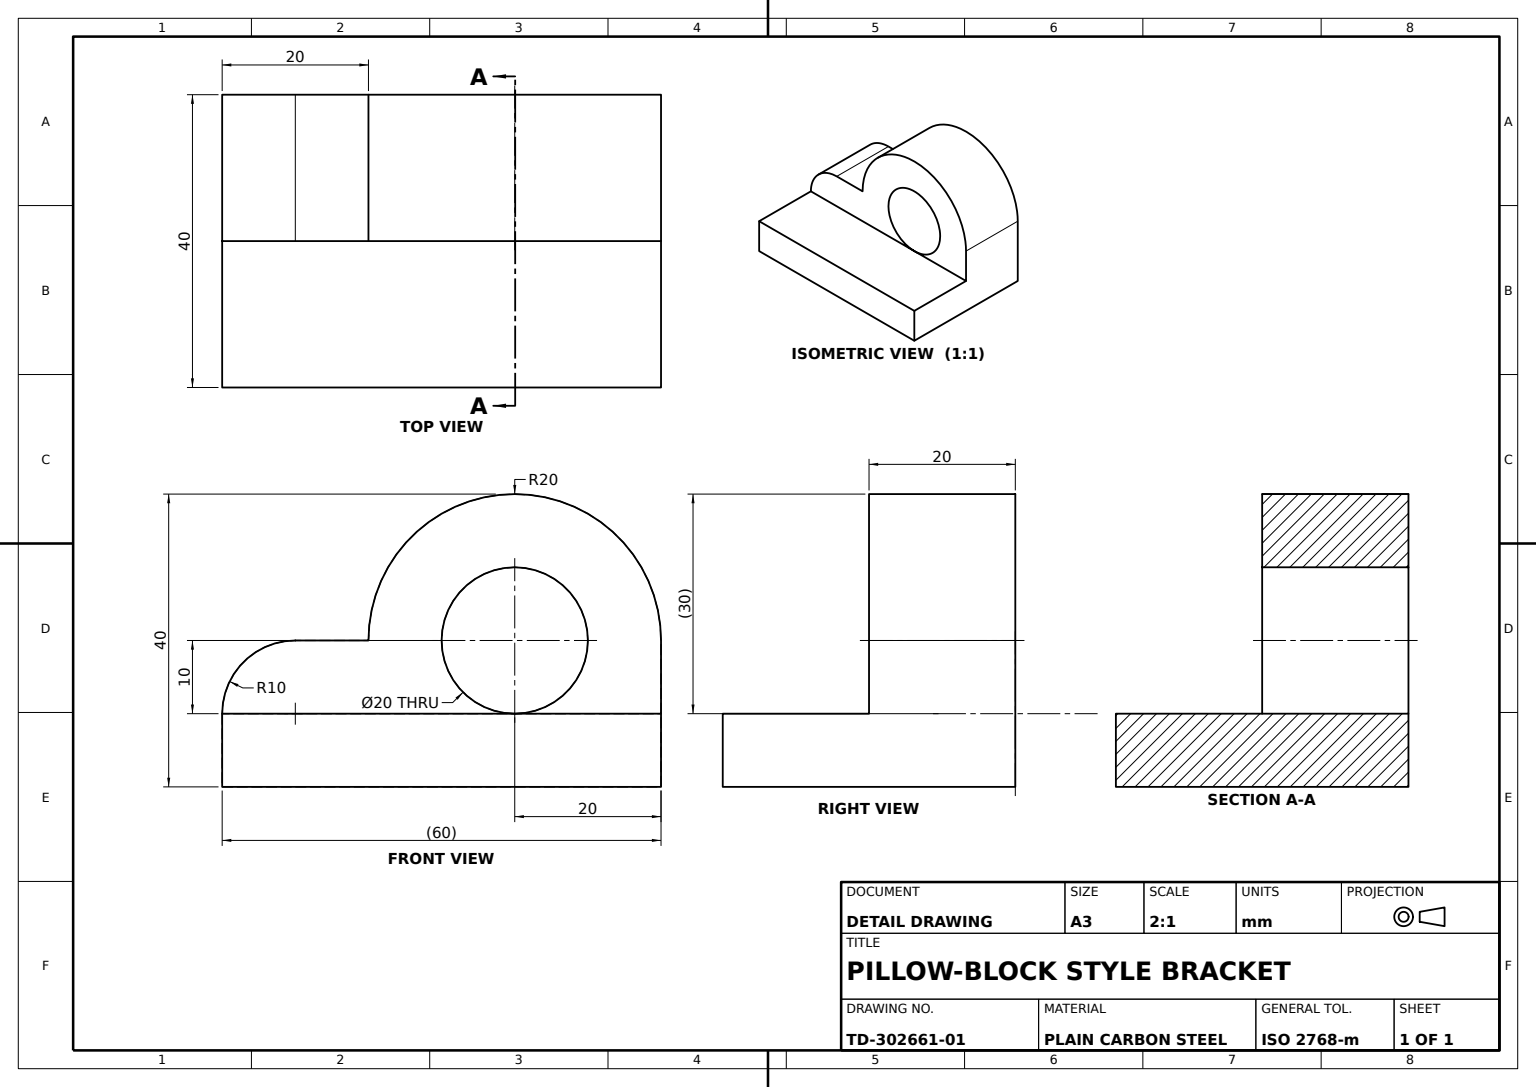
from build123d import *

# Parameters (mm, degrees)
BASE_PLATE_SKETCH_W       = 60
BASE_PLATE_SKETCH_H       = 40
BASE_PLATE_60X40X10_DEPTH = 5
UPRIGHT_LUG_SKETCH_W      = 60
UPRIGHT_LUG_SKETCH_H      = 20
UPRIGHT_LUG_DEPTH         = 30
CROSS_HOLE_SKETCH_R       = 10
CROSS_HOLE_CUT_DEPTH      = 62.032778079
LUG_PROFILE_CUT_DEPTH     = 62.032778079
LUG_ROUND_R10_R           = 10


with BuildPart() as part:
    # Base Plate Sketch → Base Plate 60x40x10 (new, symmetric)
    with BuildSketch(Plane(origin=(0, 0, 0), x_dir=(1, 0, 0), z_dir=(0, 1, 0))):
        Rectangle(BASE_PLATE_SKETCH_W, BASE_PLATE_SKETCH_H)
    extrude(amount=BASE_PLATE_60X40X10_DEPTH, both=True)

    # Upright Lug Sketch → Upright Lug (add)
    with BuildSketch(Plane(origin=(0, 5, 0), x_dir=(1, 0, 0), z_dir=(0, 1, 0))):
        with Locations((0, 10)):
            Rectangle(UPRIGHT_LUG_SKETCH_W, UPRIGHT_LUG_SKETCH_H)
    extrude(amount=UPRIGHT_LUG_DEPTH)

    # Cross Hole Sketch → Cross Hole Cut (cut, through all)
    with BuildSketch(Plane(origin=(0, 0, -20), x_dir=(-1, 0, 0), z_dir=(0, 0, -1))):
        with Locations((-10, 15)):
            Circle(CROSS_HOLE_SKETCH_R)
    extrude(amount=-CROSS_HOLE_CUT_DEPTH, mode=Mode.SUBTRACT)

    # Lug Profile Sketch → Lug Profile Cut (cut, through all)
    with BuildSketch(Plane(origin=(0, 0, -20), x_dir=(-1, 0, 0), z_dir=(0, 0, -1))):
        with BuildLine():
            Line((-30, 35), (-30, 15.000000101))
            ThreePointArc((-30, 15.000000101), (-24.142135638, 29.142135609), (-10.000000142, 35))
            Line((-10.000000142, 35), (-30, 35))
        make_face()
        with BuildLine():
            ThreePointArc((-10.000000142, 35), (4.142135574, 29.142135674), (10, 15))
            Line((10, 15), (30, 15))
            Line((30, 15), (30, 35))
            Line((30, 35), (-10.000000142, 35))
        make_face()
    extrude(amount=-LUG_PROFILE_CUT_DEPTH, mode=Mode.SUBTRACT)

    # Lug Round R10
    lug_round_r10_edges = [part.edges().sort_by_distance(p)[0] for p in [
        (-30, 15, -10),
    ]]
    fillet(lug_round_r10_edges, radius=LUG_ROUND_R10_R)


solid = part.part
